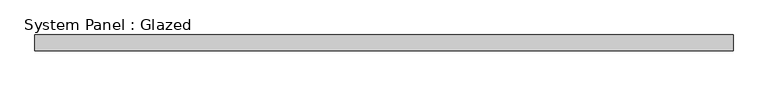
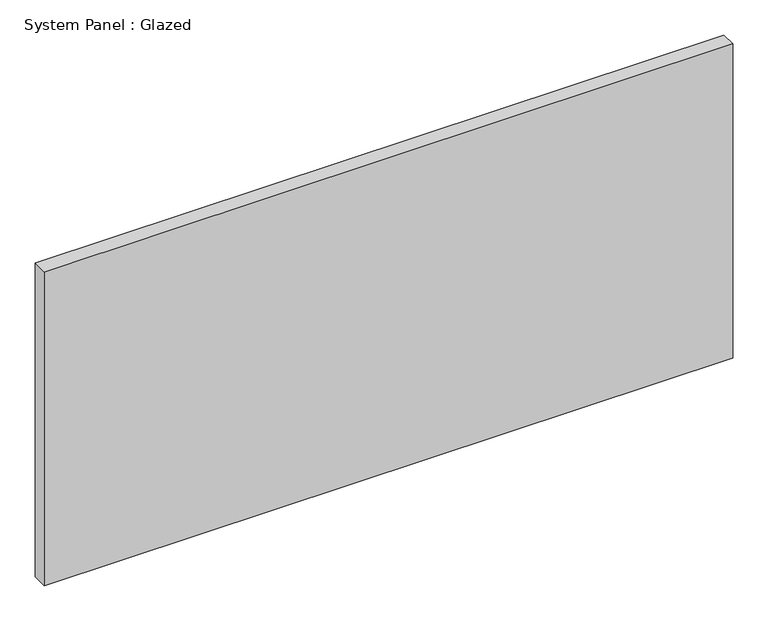
"""IFC4 building model written with IfcOpenShell, lengths in millimetres: plate geometry, System Panel : Glazed."""

from ifc_helpers import new_model, si_unit, origin, origin_with_axes, place, context, project, spatial, polyline, outline, extrude, source, transform, mapped, element, save


def system_panel_glazed_21725642(model_context):
    return source(origin(), model_context, "Body", "SweptSolid", [
        extrude(outline(polyline([(566.2083333, 19.05), (-566.2083333, 19.05), (-566.2083333, 44.45), (566.2083333, 44.45), (566.2083333, 19.05)])), origin_with_axes(), (0.0, 0.0, 1.0), 546.1),
    ])


if __name__ == "__main__":
    model = new_model("IFC4")
    model_context = context("Model", 3, world=origin())
    ifc_project = project(units=[si_unit("LENGTHUNIT", "METRE", prefix="MILLI")], contexts=[model_context])
    site = spatial("IfcSite", under=ifc_project)
    building = spatial("IfcBuilding", under=site)
    placement = place(None, origin())
    system_panel_glazed_shape = system_panel_glazed_21725642(model_context)
    element("IfcPlate", 1, ObjectType="System Panel : Glazed", at=placement, inside=building, context=model_context, shape_type="MappedRepresentation", body=[
        mapped(system_panel_glazed_shape, transform((0.0, 0.0, 0.0), x_axis=(1.0, 0.0, 0.0), y_axis=(0.0, 1.0, 0.0), z_axis=(0.0, 0.0, 1.0))),
    ])
    save(model, "model.ifc")

# Revit data of these elements
# Type "System Panel : Glazed"
#   Construction Type Id = "GSP4R"
#   Analytic Construction = "1/8 in Pilkington single glazing"
#   Visual Light Transmittance = 0.9
#   Solar Heat Gain Coefficient = 0.86
#   Heat Transfer Coefficient (U) = 1.18115 BTU/(h·ft²·°F)
# Element 1 (IfcPlate, "System Panel : Glazed")
#   Materials on its faces: "Glass"
# Materials
#   "Glass": class "Glass", colour RGB 0 128 192, transparency 0.75, Description = "Soda Lime Glass", Cost = 0
